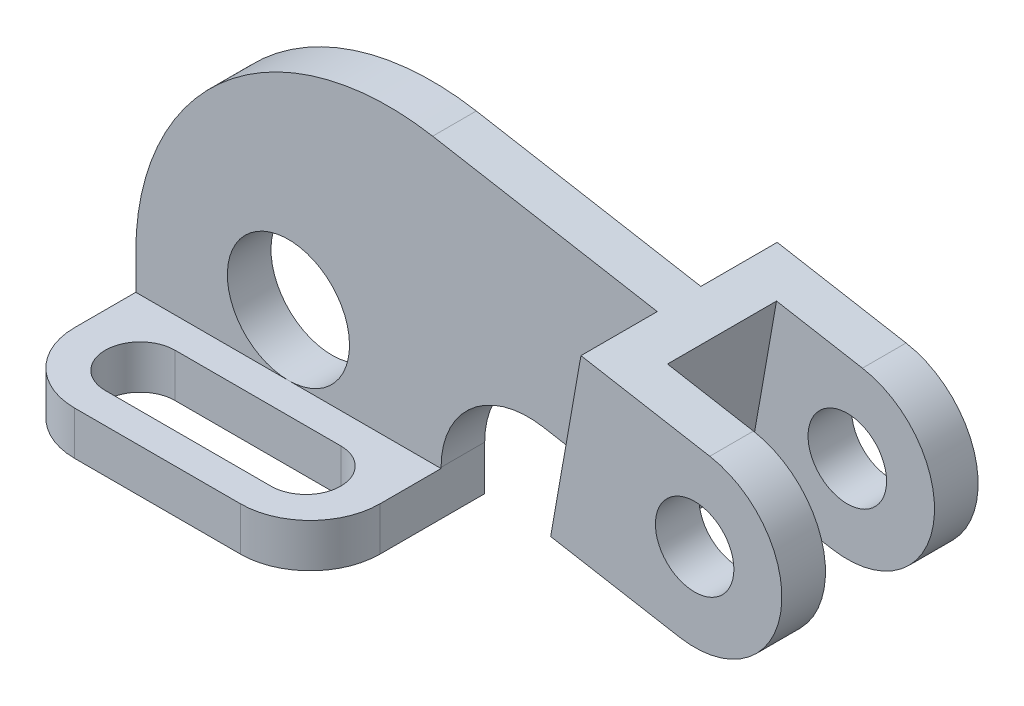
ISO-10303-21;
HEADER;
FILE_DESCRIPTION(('STEP AP214'),'2;1');
FILE_NAME('part.step','',(''),(''),'','','');
FILE_SCHEMA(('AUTOMOTIVE_DESIGN { 1 0 10303 214 1 1 1 1 }'));
ENDSEC;
DATA;
#1=APPLICATION_CONTEXT('core data for automotive mechanical design processes');
#2=APPLICATION_PROTOCOL_DEFINITION('international standard','automotive_design',2000,#1);
#3=PRODUCT_CONTEXT('',#1,'mechanical');
#4=PRODUCT('Part','Part','',(#3));
#5=PRODUCT_RELATED_PRODUCT_CATEGORY('part','',(#4));
#6=PRODUCT_DEFINITION_FORMATION('','',#4);
#7=PRODUCT_DEFINITION_CONTEXT('part definition',#1,'design');
#8=PRODUCT_DEFINITION('design','',#6,#7);
#9=PRODUCT_DEFINITION_SHAPE('','',#8);
#10=(LENGTH_UNIT() NAMED_UNIT(*) SI_UNIT(.MILLI.,.METRE.));
#11=(NAMED_UNIT(*) PLANE_ANGLE_UNIT() SI_UNIT($,.RADIAN.));
#12=(NAMED_UNIT(*) SI_UNIT($,.STERADIAN.) SOLID_ANGLE_UNIT());
#13=UNCERTAINTY_MEASURE_WITH_UNIT(LENGTH_MEASURE(1.E-05),#10,'distance_accuracy_value','');
#14=(GEOMETRIC_REPRESENTATION_CONTEXT(3) GLOBAL_UNCERTAINTY_ASSIGNED_CONTEXT((#13)) GLOBAL_UNIT_ASSIGNED_CONTEXT((#10,
#11,#12)) REPRESENTATION_CONTEXT('',''));
#15=CARTESIAN_POINT('',(0.,0.,0.));
#16=DIRECTION('',(0.,0.,1.));
#17=DIRECTION('',(1.,0.,0.));
#18=AXIS2_PLACEMENT_3D('',#15,#16,#17);
#19=CARTESIAN_POINT('',(145.640956215304,41.0463722757444,22.5));
#20=DIRECTION('',(0.,0.,1.));
#21=DIRECTION('',(1.,0.,0.));
#22=AXIS2_PLACEMENT_3D('',#19,#20,#21);
#23=CYLINDRICAL_SURFACE('',#22,20.);
#24=CARTESIAN_POINT('',(145.640956215304,41.0463722757444,-12.5));
#25=DIRECTION('',(0.,0.,-1.));
#26=DIRECTION('',(-1.,0.,0.));
#27=AXIS2_PLACEMENT_3D('',#24,#25,#26);
#28=CIRCLE('',#27,20.);
#29=CARTESIAN_POINT('',(142.167992661965,21.3502172155003,-12.5));
#30=VERTEX_POINT('',#29);
#31=CARTESIAN_POINT('',(149.113919768642,60.7425273359886,-12.5));
#32=VERTEX_POINT('',#31);
#33=EDGE_CURVE('E242',#30,#32,#28,.F.);
#34=ORIENTED_EDGE('',*,*,#33,.F.);
#35=DIRECTION('',(0.,0.,-1.));
#36=VECTOR('',#35,1.);
#37=CARTESIAN_POINT('',(142.167992661965,21.3502172155003,22.5));
#38=LINE('',#37,#36);
#39=CARTESIAN_POINT('',(142.167992661965,21.3502172155003,-22.5));
#40=VERTEX_POINT('',#39);
#41=EDGE_CURVE('E399',#40,#30,#38,.F.);
#42=ORIENTED_EDGE('',*,*,#41,.F.);
#43=CARTESIAN_POINT('',(145.640956215304,41.0463722757444,-22.5));
#44=DIRECTION('',(0.,0.,1.));
#45=DIRECTION('',(0.,-1.,0.));
#46=AXIS2_PLACEMENT_3D('',#43,#44,#45);
#47=CIRCLE('',#46,20.);
#48=CARTESIAN_POINT('',(149.113919768642,60.7425273359886,-22.5));
#49=VERTEX_POINT('',#48);
#50=EDGE_CURVE('E11',#49,#40,#47,.F.);
#51=ORIENTED_EDGE('',*,*,#50,.F.);
#52=DIRECTION('',(0.,0.,-1.));
#53=VECTOR('',#52,1.);
#54=CARTESIAN_POINT('',(149.113919768642,60.7425273359886,22.5));
#55=LINE('',#54,#53);
#56=EDGE_CURVE('E398',#32,#49,#55,.T.);
#57=ORIENTED_EDGE('',*,*,#56,.F.);
#58=EDGE_LOOP('',(#34,#42,#51,#57));
#59=FACE_BOUND('',#58,.T.);
#60=ADVANCED_FACE('F41',(#59),#23,.T.);
#61=CARTESIAN_POINT('',(68.0715943046827,75.0324758946416,5.));
#62=DIRECTION('',(-0.173648177666934,-0.984807753012207,0.));
#63=DIRECTION('',(0.984807753012207,-0.173648177666934,0.));
#64=AXIS2_PLACEMENT_3D('',#61,#62,#63);
#65=PLANE('',#64);
#66=DIRECTION('',(0.984807753012207,-0.173648177666934,0.));
#67=VECTOR('',#66,1.);
#68=CARTESIAN_POINT('',(129.417764708398,64.2154908893273,12.5));
#69=LINE('',#68,#67);
#70=CARTESIAN_POINT('',(129.417764708398,64.2154908893273,12.5));
#71=VERTEX_POINT('',#70);
#72=CARTESIAN_POINT('',(149.113919768642,60.7425273359886,12.5));
#73=VERTEX_POINT('',#72);
#74=EDGE_CURVE('E213',#71,#73,#69,.T.);
#75=ORIENTED_EDGE('',*,*,#74,.F.);
#76=DIRECTION('',(0.,0.,1.));
#77=VECTOR('',#76,1.);
#78=CARTESIAN_POINT('',(129.417764708398,64.2154908893273,-12.5));
#79=LINE('',#78,#77);
#80=CARTESIAN_POINT('',(129.417764708398,64.2154908893273,-12.5));
#81=VERTEX_POINT('',#80);
#82=EDGE_CURVE('E222',#81,#71,#79,.T.);
#83=ORIENTED_EDGE('',*,*,#82,.F.);
#84=DIRECTION('',(-0.984807753012207,0.173648177666934,0.));
#85=VECTOR('',#84,1.);
#86=CARTESIAN_POINT('',(129.417764708398,64.2154908893273,-12.5));
#87=LINE('',#86,#85);
#88=EDGE_CURVE('E56',#32,#81,#87,.T.);
#89=ORIENTED_EDGE('',*,*,#88,.F.);
#90=ORIENTED_EDGE('',*,*,#56,.T.);
#91=DIRECTION('',(-0.984807753012207,0.173648177666934,0.));
#92=VECTOR('',#91,1.);
#93=CARTESIAN_POINT('',(168.810074828886,57.2695637826499,-22.5));
#94=LINE('',#93,#92);
#95=CARTESIAN_POINT('',(119.569687178276,65.9519726659966,-22.5));
#96=VERTEX_POINT('',#95);
#97=EDGE_CURVE('E264',#49,#96,#94,.T.);
#98=ORIENTED_EDGE('',*,*,#97,.T.);
#99=DIRECTION('',(0.,0.,1.));
#100=VECTOR('',#99,1.);
#101=CARTESIAN_POINT('',(119.569687178276,65.9519726659966,22.5));
#102=LINE('',#101,#100);
#103=CARTESIAN_POINT('',(119.569687178276,65.9519726659966,-5.));
#104=VERTEX_POINT('',#103);
#105=EDGE_CURVE('E257',#96,#104,#102,.T.);
#106=ORIENTED_EDGE('',*,*,#105,.T.);
#107=DIRECTION('',(-0.984807753012207,0.173648177666934,0.));
#108=VECTOR('',#107,1.);
#109=CARTESIAN_POINT('',(68.0715943046827,75.0324758946416,-5.));
#110=LINE('',#109,#108);
#111=CARTESIAN_POINT('',(68.0715943046827,75.0324758946416,-5.));
#112=VERTEX_POINT('',#111);
#113=EDGE_CURVE('E373',#104,#112,#110,.T.);
#114=ORIENTED_EDGE('',*,*,#113,.T.);
#115=DIRECTION('',(0.,0.,-1.));
#116=VECTOR('',#115,1.);
#117=CARTESIAN_POINT('',(68.0715943046827,75.0324758946416,5.));
#118=LINE('',#117,#116);
#119=CARTESIAN_POINT('',(68.0715943046827,75.0324758946416,5.));
#120=VERTEX_POINT('',#119);
#121=EDGE_CURVE('E382',#120,#112,#118,.T.);
#122=ORIENTED_EDGE('',*,*,#121,.F.);
#123=DIRECTION('',(-0.984807753012207,0.173648177666934,0.));
#124=VECTOR('',#123,1.);
#125=CARTESIAN_POINT('',(68.0715943046827,75.0324758946416,5.));
#126=LINE('',#125,#124);
#127=CARTESIAN_POINT('',(119.569687178276,65.9519726659966,5.));
#128=VERTEX_POINT('',#127);
#129=EDGE_CURVE('E351',#128,#120,#126,.T.);
#130=ORIENTED_EDGE('',*,*,#129,.F.);
#131=CARTESIAN_POINT('',(119.569687178276,65.9519726659966,22.5));
#132=VERTEX_POINT('',#131);
#133=EDGE_CURVE('E259',#128,#132,#102,.T.);
#134=ORIENTED_EDGE('',*,*,#133,.T.);
#135=DIRECTION('',(-0.984807753012207,0.173648177666934,0.));
#136=VECTOR('',#135,1.);
#137=CARTESIAN_POINT('',(168.810074828886,57.2695637826499,22.5));
#138=LINE('',#137,#136);
#139=CARTESIAN_POINT('',(149.113919768642,60.7425273359886,22.5));
#140=VERTEX_POINT('',#139);
#141=EDGE_CURVE('E263',#140,#132,#138,.T.);
#142=ORIENTED_EDGE('',*,*,#141,.F.);
#143=EDGE_CURVE('E229',#140,#73,#55,.T.);
#144=ORIENTED_EDGE('',*,*,#143,.T.);
#145=EDGE_LOOP('',(#75,#83,#89,#90,#98,#106,#114,#122,#130,#134,#142,#144));
#146=FACE_BOUND('',#145,.T.);
#147=ADVANCED_FACE('F227',(#146),#65,.F.);
#148=CARTESIAN_POINT('',(145.640956215304,41.0463722757444,-27.5));
#149=DIRECTION('',(0.,0.,1.));
#150=DIRECTION('',(1.,0.,0.));
#151=AXIS2_PLACEMENT_3D('',#148,#149,#150);
#152=CYLINDRICAL_SURFACE('',#151,9.00000000000001);
#153=CARTESIAN_POINT('',(145.640956215304,41.0463722757444,-12.5));
#154=DIRECTION('',(0.,0.,-1.));
#155=DIRECTION('',(-1.,0.,0.));
#156=AXIS2_PLACEMENT_3D('',#153,#154,#155);
#157=CIRCLE('',#156,9.00000000000001);
#158=CARTESIAN_POINT('',(154.640956215304,41.0463722757444,-12.5));
#159=VERTEX_POINT('',#158);
#160=EDGE_CURVE('E46',#159,#159,#157,.F.);
#161=CARTESIAN_POINT('',(145.640956215304,41.0463722757444,-22.5));
#162=DIRECTION('',(0.,0.,1.));
#163=DIRECTION('',(0.,-1.,0.));
#164=AXIS2_PLACEMENT_3D('',#161,#162,#163);
#165=CIRCLE('',#164,9.00000000000001);
#166=CARTESIAN_POINT('',(154.640956215304,41.0463722757444,-22.5));
#167=VERTEX_POINT('',#166);
#168=EDGE_CURVE('E247',#167,#167,#165,.T.);
#169=CARTESIAN_POINT('',(154.640956215304,41.0463722757444,-12.5));
#170=CARTESIAN_POINT('',(154.640956215304,41.0463722757444,-12.6041666666667));
#171=CARTESIAN_POINT('',(154.640956215304,41.0463722757444,-12.7083333333333));
#172=CARTESIAN_POINT('',(154.640956215304,41.0463722757444,-12.9166666666667));
#173=CARTESIAN_POINT('',(154.640956215304,41.0463722757444,-13.0208333333333));
#174=CARTESIAN_POINT('',(154.640956215304,41.0463722757444,-13.2291666666667));
#175=CARTESIAN_POINT('',(154.640956215304,41.0463722757444,-13.3333333333333));
#176=CARTESIAN_POINT('',(154.640956215304,41.0463722757444,-13.5416666666667));
#177=CARTESIAN_POINT('',(154.640956215304,41.0463722757444,-13.6458333333333));
#178=CARTESIAN_POINT('',(154.640956215304,41.0463722757444,-13.8541666666667));
#179=CARTESIAN_POINT('',(154.640956215304,41.0463722757444,-13.9583333333333));
#180=CARTESIAN_POINT('',(154.640956215304,41.0463722757444,-14.1666666666667));
#181=CARTESIAN_POINT('',(154.640956215304,41.0463722757444,-14.2708333333333));
#182=CARTESIAN_POINT('',(154.640956215304,41.0463722757444,-14.4791666666667));
#183=CARTESIAN_POINT('',(154.640956215304,41.0463722757444,-14.5833333333333));
#184=CARTESIAN_POINT('',(154.640956215304,41.0463722757444,-14.7916666666667));
#185=CARTESIAN_POINT('',(154.640956215304,41.0463722757444,-14.8958333333333));
#186=CARTESIAN_POINT('',(154.640956215304,41.0463722757444,-15.1041666666667));
#187=CARTESIAN_POINT('',(154.640956215304,41.0463722757444,-15.2083333333333));
#188=CARTESIAN_POINT('',(154.640956215304,41.0463722757444,-15.4166666666667));
#189=CARTESIAN_POINT('',(154.640956215304,41.0463722757444,-15.5208333333333));
#190=CARTESIAN_POINT('',(154.640956215304,41.0463722757444,-15.7291666666667));
#191=CARTESIAN_POINT('',(154.640956215304,41.0463722757444,-15.8333333333333));
#192=CARTESIAN_POINT('',(154.640956215304,41.0463722757444,-16.0416666666667));
#193=CARTESIAN_POINT('',(154.640956215304,41.0463722757444,-16.1458333333333));
#194=CARTESIAN_POINT('',(154.640956215304,41.0463722757444,-16.3541666666667));
#195=CARTESIAN_POINT('',(154.640956215304,41.0463722757444,-16.4583333333333));
#196=CARTESIAN_POINT('',(154.640956215304,41.0463722757444,-16.6666666666667));
#197=CARTESIAN_POINT('',(154.640956215304,41.0463722757444,-16.7708333333333));
#198=CARTESIAN_POINT('',(154.640956215304,41.0463722757444,-16.9791666666667));
#199=CARTESIAN_POINT('',(154.640956215304,41.0463722757444,-17.0833333333333));
#200=CARTESIAN_POINT('',(154.640956215304,41.0463722757444,-17.2916666666667));
#201=CARTESIAN_POINT('',(154.640956215304,41.0463722757444,-17.3958333333333));
#202=CARTESIAN_POINT('',(154.640956215304,41.0463722757444,-17.6041666666667));
#203=CARTESIAN_POINT('',(154.640956215304,41.0463722757444,-17.7083333333333));
#204=CARTESIAN_POINT('',(154.640956215304,41.0463722757444,-17.9166666666667));
#205=CARTESIAN_POINT('',(154.640956215304,41.0463722757444,-18.0208333333333));
#206=CARTESIAN_POINT('',(154.640956215304,41.0463722757444,-18.2291666666667));
#207=CARTESIAN_POINT('',(154.640956215304,41.0463722757444,-18.3333333333333));
#208=CARTESIAN_POINT('',(154.640956215304,41.0463722757444,-18.5416666666667));
#209=CARTESIAN_POINT('',(154.640956215304,41.0463722757444,-18.6458333333333));
#210=CARTESIAN_POINT('',(154.640956215304,41.0463722757444,-18.8541666666667));
#211=CARTESIAN_POINT('',(154.640956215304,41.0463722757444,-18.9583333333333));
#212=CARTESIAN_POINT('',(154.640956215304,41.0463722757444,-19.1666666666667));
#213=CARTESIAN_POINT('',(154.640956215304,41.0463722757444,-19.2708333333333));
#214=CARTESIAN_POINT('',(154.640956215304,41.0463722757444,-19.4791666666667));
#215=CARTESIAN_POINT('',(154.640956215304,41.0463722757444,-19.5833333333333));
#216=CARTESIAN_POINT('',(154.640956215304,41.0463722757444,-19.7916666666667));
#217=CARTESIAN_POINT('',(154.640956215304,41.0463722757444,-19.8958333333333));
#218=CARTESIAN_POINT('',(154.640956215304,41.0463722757444,-20.1041666666667));
#219=CARTESIAN_POINT('',(154.640956215304,41.0463722757444,-20.2083333333333));
#220=CARTESIAN_POINT('',(154.640956215304,41.0463722757444,-20.4166666666667));
#221=CARTESIAN_POINT('',(154.640956215304,41.0463722757444,-20.5208333333333));
#222=CARTESIAN_POINT('',(154.640956215304,41.0463722757444,-20.7291666666667));
#223=CARTESIAN_POINT('',(154.640956215304,41.0463722757444,-20.8333333333333));
#224=CARTESIAN_POINT('',(154.640956215304,41.0463722757444,-21.0416666666667));
#225=CARTESIAN_POINT('',(154.640956215304,41.0463722757444,-21.1458333333333));
#226=CARTESIAN_POINT('',(154.640956215304,41.0463722757444,-21.3541666666667));
#227=CARTESIAN_POINT('',(154.640956215304,41.0463722757444,-21.4583333333333));
#228=CARTESIAN_POINT('',(154.640956215304,41.0463722757444,-21.6666666666667));
#229=CARTESIAN_POINT('',(154.640956215304,41.0463722757444,-21.7708333333333));
#230=CARTESIAN_POINT('',(154.640956215304,41.0463722757444,-21.9791666666667));
#231=CARTESIAN_POINT('',(154.640956215304,41.0463722757444,-22.0833333333333));
#232=CARTESIAN_POINT('',(154.640956215304,41.0463722757444,-22.2916666666667));
#233=CARTESIAN_POINT('',(154.640956215304,41.0463722757444,-22.3958333333333));
#234=CARTESIAN_POINT('',(154.640956215304,41.0463722757444,-22.5));
#235=B_SPLINE_CURVE_WITH_KNOTS('',3,(#169,#170,#171,#172,#173,#174,#175,#176,#177,#178,#179,
#180,#181,#182,#183,#184,#185,#186,#187,#188,#189,#190,#191,#192,#193,#194,#195,#196,#197,#198,
#199,#200,#201,#202,#203,#204,#205,#206,#207,#208,#209,#210,#211,#212,#213,#214,#215,#216,#217,
#218,#219,#220,#221,#222,#223,#224,#225,#226,#227,#228,#229,#230,#231,#232,#233,#234),
.UNSPECIFIED.,.F.,.F.,(4,2,2,2,2,2,2,2,2,2,2,2,2,2,2,2,2,2,2,2,2,2,2,2,2,2,2,2,2,2,2,2,4),(0.,
0.3125,0.625000000000001,0.937500000000001,1.25,1.5625,1.875,2.1875,2.5,2.8125,3.125,3.4375,
3.75,4.0625,4.375,4.6875,5.,5.3125,5.62500000000001,5.93750000000001,6.25000000000001,
6.56250000000001,6.87500000000001,7.18750000000001,7.5,7.8125,8.125,8.4375,8.75,
9.06250000000001,9.37500000000001,9.68750000000001,10.),.UNSPECIFIED.);
#236=EDGE_CURVE('BSEAM423',#159,#167,#235,.T.);
#237=ORIENTED_EDGE('',*,*,#160,.T.);
#238=ORIENTED_EDGE('',*,*,#168,.F.);
#239=ORIENTED_EDGE('',*,*,#236,.T.);
#240=ORIENTED_EDGE('',*,*,#236,.F.);
#241=EDGE_LOOP('',(#237,#239,#238,#240));
#242=FACE_BOUND('',#241,.T.);
#243=ADVANCED_FACE('F423',(#242),#152,.F.);
#244=CARTESIAN_POINT('',(145.640956215304,41.0463722757444,12.5));
#245=DIRECTION('',(0.,0.,1.));
#246=DIRECTION('',(1.,0.,0.));
#247=AXIS2_PLACEMENT_3D('',#244,#245,#246);
#248=CIRCLE('',#247,20.);
#249=CARTESIAN_POINT('',(142.167992661965,21.3502172155003,12.5));
#250=VERTEX_POINT('',#249);
#251=EDGE_CURVE('E237',#73,#250,#248,.F.);
#252=ORIENTED_EDGE('',*,*,#251,.F.);
#253=ORIENTED_EDGE('',*,*,#143,.F.);
#254=CARTESIAN_POINT('',(145.640956215304,41.0463722757444,22.5));
#255=DIRECTION('',(0.,0.,-1.));
#256=DIRECTION('',(0.,1.,0.));
#257=AXIS2_PLACEMENT_3D('',#254,#255,#256);
#258=CIRCLE('',#257,20.);
#259=CARTESIAN_POINT('',(142.167992661965,21.3502172155003,22.5));
#260=VERTEX_POINT('',#259);
#261=EDGE_CURVE('E51',#260,#140,#258,.F.);
#262=ORIENTED_EDGE('',*,*,#261,.F.);
#263=EDGE_CURVE('E69',#250,#260,#38,.F.);
#264=ORIENTED_EDGE('',*,*,#263,.F.);
#265=EDGE_LOOP('',(#252,#253,#262,#264));
#266=FACE_BOUND('',#265,.T.);
#267=ADVANCED_FACE('F42',(#266),#23,.T.);
#268=CARTESIAN_POINT('',(58.,17.9136262199337,5.));
#269=DIRECTION('',(0.,0.,1.));
#270=DIRECTION('',(1.,0.,0.));
#271=AXIS2_PLACEMENT_3D('',#268,#269,#270);
#272=PLANE('',#271);
#273=DIRECTION('',(-1.,0.,0.));
#274=VECTOR('',#273,1.);
#275=CARTESIAN_POINT('',(0.,10.,5.));
#276=LINE('',#275,#274);
#277=CARTESIAN_POINT('',(70.,10.,5.));
#278=VERTEX_POINT('',#277);
#279=CARTESIAN_POINT('',(35.,10.,5.));
#280=VERTEX_POINT('',#279);
#281=EDGE_CURVE('E316',#278,#280,#276,.T.);
#282=ORIENTED_EDGE('',*,*,#281,.F.);
#283=DIRECTION('',(0.,1.,0.));
#284=VECTOR('',#283,1.);
#285=CARTESIAN_POINT('',(70.,10.240309613491,5.));
#286=LINE('',#285,#284);
#287=CARTESIAN_POINT('',(70.,10.240309613491,5.));
#288=VERTEX_POINT('',#287);
#289=EDGE_CURVE('E345',#278,#288,#286,.T.);
#290=ORIENTED_EDGE('',*,*,#289,.T.);
#291=CARTESIAN_POINT('',(90.,10.2403096134912,5.));
#292=DIRECTION('',(0.,0.,-1.));
#293=DIRECTION('',(1.,0.,0.));
#294=AXIS2_PLACEMENT_3D('',#291,#292,#293);
#295=CIRCLE('',#294,20.);
#296=CARTESIAN_POINT('',(93.4729635533388,29.9364646737353,5.));
#297=VERTEX_POINT('',#296);
#298=EDGE_CURVE('E347',#288,#297,#295,.T.);
#299=ORIENTED_EDGE('',*,*,#298,.T.);
#300=DIRECTION('',(0.984807753012207,-0.173648177666934,0.));
#301=VECTOR('',#300,1.);
#302=CARTESIAN_POINT('',(112.623760071599,26.5596625455083,5.));
#303=LINE('',#302,#301);
#304=CARTESIAN_POINT('',(112.623760071599,26.5596625455083,5.00000000000001));
#305=VERTEX_POINT('',#304);
#306=EDGE_CURVE('E349',#297,#305,#303,.T.);
#307=ORIENTED_EDGE('',*,*,#306,.T.);
#308=DIRECTION('',(0.173648177666934,0.984807753012207,0.));
#309=VECTOR('',#308,1.);
#310=CARTESIAN_POINT('',(119.569687178276,65.9519726659966,5.));
#311=LINE('',#310,#309);
#312=EDGE_CURVE('E355',#305,#128,#311,.T.);
#313=ORIENTED_EDGE('',*,*,#312,.T.);
#314=ORIENTED_EDGE('',*,*,#129,.T.);
#315=CARTESIAN_POINT('',(58.,17.9136262199337,5.));
#316=DIRECTION('',(0.,0.,1.));
#317=DIRECTION('',(1.,0.,0.));
#318=AXIS2_PLACEMENT_3D('',#315,#316,#317);
#319=CIRCLE('',#318,58.);
#320=CARTESIAN_POINT('',(0.,17.9136262199332,5.));
#321=VERTEX_POINT('',#320);
#322=EDGE_CURVE('E359',#120,#321,#319,.T.);
#323=ORIENTED_EDGE('',*,*,#322,.T.);
#324=DIRECTION('',(0.,-1.,0.));
#325=VECTOR('',#324,1.);
#326=CARTESIAN_POINT('',(0.,0.,5.));
#327=LINE('',#326,#325);
#328=CARTESIAN_POINT('',(0.,10.,5.));
#329=VERTEX_POINT('',#328);
#330=EDGE_CURVE('E360',#321,#329,#327,.T.);
#331=ORIENTED_EDGE('',*,*,#330,.T.);
#332=EDGE_CURVE('E319',#280,#329,#276,.T.);
#333=ORIENTED_EDGE('',*,*,#332,.F.);
#334=CARTESIAN_POINT('',(35.,24.,5.));
#335=DIRECTION('',(0.,0.,1.));
#336=DIRECTION('',(1.,0.,0.));
#337=AXIS2_PLACEMENT_3D('',#334,#335,#336);
#338=CIRCLE('',#337,14.);
#339=EDGE_CURVE('E338',#280,#280,#338,.T.);
#340=ORIENTED_EDGE('',*,*,#339,.F.);
#341=EDGE_LOOP('',(#282,#290,#299,#307,#313,#314,#323,#331,#333,#340));
#342=FACE_BOUND('',#341,.T.);
#343=ADVANCED_FACE('F422',(#342),#272,.T.);
#344=CARTESIAN_POINT('',(58.,17.9136262199337,-5.));
#345=DIRECTION('',(0.,0.,1.));
#346=DIRECTION('',(1.,0.,0.));
#347=AXIS2_PLACEMENT_3D('',#344,#345,#346);
#348=PLANE('',#347);
#349=DIRECTION('',(1.,0.,0.));
#350=VECTOR('',#349,1.);
#351=CARTESIAN_POINT('',(70.,0.,-5.));
#352=LINE('',#351,#350);
#353=CARTESIAN_POINT('',(0.,0.,-5.));
#354=VERTEX_POINT('',#353);
#355=CARTESIAN_POINT('',(70.,0.,-5.));
#356=VERTEX_POINT('',#355);
#357=EDGE_CURVE('E343',#354,#356,#352,.T.);
#358=ORIENTED_EDGE('',*,*,#357,.F.);
#359=DIRECTION('',(0.,-1.,0.));
#360=VECTOR('',#359,1.);
#361=CARTESIAN_POINT('',(0.,0.,-5.));
#362=LINE('',#361,#360);
#363=CARTESIAN_POINT('',(0.,17.9136262199332,-5.));
#364=VERTEX_POINT('',#363);
#365=EDGE_CURVE('E350',#364,#354,#362,.T.);
#366=ORIENTED_EDGE('',*,*,#365,.F.);
#367=CARTESIAN_POINT('',(58.,17.9136262199337,-5.));
#368=DIRECTION('',(0.,0.,1.));
#369=DIRECTION('',(1.,0.,0.));
#370=AXIS2_PLACEMENT_3D('',#367,#368,#369);
#371=CIRCLE('',#370,58.);
#372=EDGE_CURVE('E374',#112,#364,#371,.T.);
#373=ORIENTED_EDGE('',*,*,#372,.F.);
#374=ORIENTED_EDGE('',*,*,#113,.F.);
#375=DIRECTION('',(0.173648177666934,0.984807753012207,0.));
#376=VECTOR('',#375,1.);
#377=CARTESIAN_POINT('',(119.569687178276,65.9519726659966,-5.));
#378=LINE('',#377,#376);
#379=CARTESIAN_POINT('',(112.623760071599,26.5596625455083,-4.99999999999999));
#380=VERTEX_POINT('',#379);
#381=EDGE_CURVE('E371',#380,#104,#378,.T.);
#382=ORIENTED_EDGE('',*,*,#381,.F.);
#383=DIRECTION('',(0.984807753012207,-0.173648177666934,0.));
#384=VECTOR('',#383,1.);
#385=CARTESIAN_POINT('',(112.623760071599,26.5596625455083,-5.));
#386=LINE('',#385,#384);
#387=CARTESIAN_POINT('',(93.4729635533388,29.9364646737353,-5.));
#388=VERTEX_POINT('',#387);
#389=EDGE_CURVE('E366',#388,#380,#386,.T.);
#390=ORIENTED_EDGE('',*,*,#389,.F.);
#391=CARTESIAN_POINT('',(90.,10.2403096134912,-5.));
#392=DIRECTION('',(0.,0.,-1.));
#393=DIRECTION('',(1.,0.,0.));
#394=AXIS2_PLACEMENT_3D('',#391,#392,#393);
#395=CIRCLE('',#394,20.);
#396=CARTESIAN_POINT('',(70.,10.240309613491,-5.));
#397=VERTEX_POINT('',#396);
#398=EDGE_CURVE('E368',#397,#388,#395,.T.);
#399=ORIENTED_EDGE('',*,*,#398,.F.);
#400=DIRECTION('',(0.,1.,0.));
#401=VECTOR('',#400,1.);
#402=CARTESIAN_POINT('',(70.,10.240309613491,-5.));
#403=LINE('',#402,#401);
#404=EDGE_CURVE('E365',#356,#397,#403,.T.);
#405=ORIENTED_EDGE('',*,*,#404,.F.);
#406=EDGE_LOOP('',(#358,#366,#373,#374,#382,#390,#399,#405));
#407=FACE_BOUND('',#406,.T.);
#408=CARTESIAN_POINT('',(35.,24.,-5.));
#409=DIRECTION('',(0.,0.,1.));
#410=DIRECTION('',(1.,0.,0.));
#411=AXIS2_PLACEMENT_3D('',#408,#409,#410);
#412=CIRCLE('',#411,14.);
#413=CARTESIAN_POINT('',(49.,24.,-5.));
#414=VERTEX_POINT('',#413);
#415=EDGE_CURVE('E340',#414,#414,#412,.T.);
#416=ORIENTED_EDGE('',*,*,#415,.T.);
#417=EDGE_LOOP('',(#416));
#418=FACE_BOUND('',#417,.T.);
#419=ADVANCED_FACE('F435',(#407,#418),#348,.F.);
#420=CARTESIAN_POINT('',(70.,0.,5.));
#421=DIRECTION('',(0.,1.,0.));
#422=DIRECTION('',(0.,0.,1.));
#423=AXIS2_PLACEMENT_3D('',#420,#421,#422);
#424=PLANE('',#423);
#425=ORIENTED_EDGE('',*,*,#357,.T.);
#426=DIRECTION('',(0.,0.,-1.));
#427=VECTOR('',#426,1.);
#428=CARTESIAN_POINT('',(70.,0.,5.));
#429=LINE('',#428,#427);
#430=CARTESIAN_POINT('',(70.,0.,19.));
#431=VERTEX_POINT('',#430);
#432=EDGE_CURVE('E395',#431,#356,#429,.T.);
#433=ORIENTED_EDGE('',*,*,#432,.F.);
#434=CARTESIAN_POINT('',(54.,0.,19.));
#435=DIRECTION('',(0.,1.,0.));
#436=DIRECTION('',(0.,0.,-1.));
#437=AXIS2_PLACEMENT_3D('',#434,#435,#436);
#438=CIRCLE('',#437,16.);
#439=CARTESIAN_POINT('',(54.,0.,35.));
#440=VERTEX_POINT('',#439);
#441=EDGE_CURVE('E307',#440,#431,#438,.T.);
#442=ORIENTED_EDGE('',*,*,#441,.F.);
#443=DIRECTION('',(1.,0.,0.));
#444=VECTOR('',#443,1.);
#445=CARTESIAN_POINT('',(16.,0.,35.));
#446=LINE('',#445,#444);
#447=CARTESIAN_POINT('',(16.,0.,35.));
#448=VERTEX_POINT('',#447);
#449=EDGE_CURVE('E325',#448,#440,#446,.T.);
#450=ORIENTED_EDGE('',*,*,#449,.F.);
#451=CARTESIAN_POINT('',(16.,0.,19.));
#452=DIRECTION('',(0.,1.,0.));
#453=DIRECTION('',(0.,0.,-1.));
#454=AXIS2_PLACEMENT_3D('',#451,#452,#453);
#455=CIRCLE('',#454,16.);
#456=CARTESIAN_POINT('',(0.,0.,19.));
#457=VERTEX_POINT('',#456);
#458=EDGE_CURVE('E304',#457,#448,#455,.T.);
#459=ORIENTED_EDGE('',*,*,#458,.F.);
#460=DIRECTION('',(0.,0.,-1.));
#461=VECTOR('',#460,1.);
#462=CARTESIAN_POINT('',(0.,0.,5.));
#463=LINE('',#462,#461);
#464=EDGE_CURVE('E363',#457,#354,#463,.T.);
#465=ORIENTED_EDGE('',*,*,#464,.T.);
#466=EDGE_LOOP('',(#425,#433,#442,#450,#459,#465));
#467=FACE_BOUND('',#466,.T.);
#468=DIRECTION('',(-1.,0.,0.));
#469=VECTOR('',#468,1.);
#470=CARTESIAN_POINT('',(16.,0.,12.));
#471=LINE('',#470,#469);
#472=CARTESIAN_POINT('',(54.,0.,12.));
#473=VERTEX_POINT('',#472);
#474=CARTESIAN_POINT('',(16.,0.,12.));
#475=VERTEX_POINT('',#474);
#476=EDGE_CURVE('E274',#473,#475,#471,.T.);
#477=ORIENTED_EDGE('',*,*,#476,.T.);
#478=CARTESIAN_POINT('',(16.,0.,20.));
#479=DIRECTION('',(0.,1.,0.));
#480=DIRECTION('',(0.,0.,1.));
#481=AXIS2_PLACEMENT_3D('',#478,#479,#480);
#482=CIRCLE('',#481,8.);
#483=CARTESIAN_POINT('',(16.,0.,28.));
#484=VERTEX_POINT('',#483);
#485=EDGE_CURVE('E271',#475,#484,#482,.T.);
#486=ORIENTED_EDGE('',*,*,#485,.T.);
#487=DIRECTION('',(1.,0.,0.));
#488=VECTOR('',#487,1.);
#489=CARTESIAN_POINT('',(16.,0.,28.));
#490=LINE('',#489,#488);
#491=CARTESIAN_POINT('',(54.,0.,28.));
#492=VERTEX_POINT('',#491);
#493=EDGE_CURVE('E281',#484,#492,#490,.T.);
#494=ORIENTED_EDGE('',*,*,#493,.T.);
#495=CARTESIAN_POINT('',(54.,0.,20.));
#496=DIRECTION('',(0.,1.,0.));
#497=DIRECTION('',(0.,0.,1.));
#498=AXIS2_PLACEMENT_3D('',#495,#496,#497);
#499=CIRCLE('',#498,8.);
#500=EDGE_CURVE('E287',#492,#473,#499,.T.);
#501=ORIENTED_EDGE('',*,*,#500,.T.);
#502=EDGE_LOOP('',(#477,#486,#494,#501));
#503=FACE_BOUND('',#502,.T.);
#504=ADVANCED_FACE('F487',(#467,#503),#424,.F.);
#505=CARTESIAN_POINT('',(70.,10.240309613491,5.));
#506=DIRECTION('',(-1.,0.,0.));
#507=DIRECTION('',(0.,0.,1.));
#508=AXIS2_PLACEMENT_3D('',#505,#506,#507);
#509=PLANE('',#508);
#510=ORIENTED_EDGE('',*,*,#404,.T.);
#511=DIRECTION('',(0.,0.,-1.));
#512=VECTOR('',#511,1.);
#513=CARTESIAN_POINT('',(70.,10.240309613491,5.));
#514=LINE('',#513,#512);
#515=EDGE_CURVE('E386',#288,#397,#514,.T.);
#516=ORIENTED_EDGE('',*,*,#515,.F.);
#517=ORIENTED_EDGE('',*,*,#289,.F.);
#518=DIRECTION('',(0.,0.,-1.));
#519=VECTOR('',#518,1.);
#520=CARTESIAN_POINT('',(70.,10.,5.));
#521=LINE('',#520,#519);
#522=CARTESIAN_POINT('',(70.,10.,19.));
#523=VERTEX_POINT('',#522);
#524=EDGE_CURVE('E311',#523,#278,#521,.T.);
#525=ORIENTED_EDGE('',*,*,#524,.F.);
#526=DIRECTION('',(0.,-1.,0.));
#527=VECTOR('',#526,1.);
#528=CARTESIAN_POINT('',(70.,10.,19.));
#529=LINE('',#528,#527);
#530=EDGE_CURVE('E317',#523,#431,#529,.T.);
#531=ORIENTED_EDGE('',*,*,#530,.T.);
#532=ORIENTED_EDGE('',*,*,#432,.T.);
#533=EDGE_LOOP('',(#510,#516,#517,#525,#531,#532));
#534=FACE_BOUND('',#533,.T.);
#535=ADVANCED_FACE('F480',(#534),#509,.F.);
#536=CARTESIAN_POINT('',(90.,10.2403096134912,5.));
#537=DIRECTION('',(0.,0.,-1.));
#538=DIRECTION('',(-1.,0.,0.));
#539=AXIS2_PLACEMENT_3D('',#536,#537,#538);
#540=CYLINDRICAL_SURFACE('',#539,20.);
#541=ORIENTED_EDGE('',*,*,#398,.T.);
#542=DIRECTION('',(0.,0.,-1.));
#543=VECTOR('',#542,1.);
#544=CARTESIAN_POINT('',(93.4729635533388,29.9364646737353,5.));
#545=LINE('',#544,#543);
#546=EDGE_CURVE('E387',#297,#388,#545,.T.);
#547=ORIENTED_EDGE('',*,*,#546,.F.);
#548=ORIENTED_EDGE('',*,*,#298,.F.);
#549=ORIENTED_EDGE('',*,*,#515,.T.);
#550=EDGE_LOOP('',(#541,#547,#548,#549));
#551=FACE_BOUND('',#550,.T.);
#552=ADVANCED_FACE('F508',(#551),#540,.F.);
#553=CARTESIAN_POINT('',(112.623760071599,26.5596625455083,5.));
#554=DIRECTION('',(0.173648177666934,0.984807753012207,0.));
#555=DIRECTION('',(-0.984807753012208,0.173648177666934,0.));
#556=AXIS2_PLACEMENT_3D('',#553,#554,#555);
#557=PLANE('',#556);
#558=ORIENTED_EDGE('',*,*,#41,.T.);
#559=DIRECTION('',(-0.984807753012207,0.173648177666934,0.));
#560=VECTOR('',#559,1.);
#561=CARTESIAN_POINT('',(112.623760071599,26.5596625455083,-12.5));
#562=LINE('',#561,#560);
#563=CARTESIAN_POINT('',(122.471837601721,24.823180768839,-12.5));
#564=VERTEX_POINT('',#563);
#565=EDGE_CURVE('E236',#30,#564,#562,.T.);
#566=ORIENTED_EDGE('',*,*,#565,.T.);
#567=DIRECTION('',(0.,0.,1.));
#568=VECTOR('',#567,1.);
#569=CARTESIAN_POINT('',(122.471837601721,24.8231807688389,5.));
#570=LINE('',#569,#568);
#571=CARTESIAN_POINT('',(122.471837601721,24.823180768839,12.5));
#572=VERTEX_POINT('',#571);
#573=EDGE_CURVE('E243',#564,#572,#570,.T.);
#574=ORIENTED_EDGE('',*,*,#573,.T.);
#575=DIRECTION('',(0.984807753012207,-0.173648177666934,0.));
#576=VECTOR('',#575,1.);
#577=CARTESIAN_POINT('',(112.623760071599,26.5596625455083,12.5));
#578=LINE('',#577,#576);
#579=EDGE_CURVE('E214',#572,#250,#578,.T.);
#580=ORIENTED_EDGE('',*,*,#579,.T.);
#581=ORIENTED_EDGE('',*,*,#263,.T.);
#582=DIRECTION('',(-0.984807753012207,0.173648177666934,0.));
#583=VECTOR('',#582,1.);
#584=CARTESIAN_POINT('',(161.864147722209,17.8772536621616,22.5));
#585=LINE('',#584,#583);
#586=CARTESIAN_POINT('',(112.623760071599,26.5596625455083,22.5));
#587=VERTEX_POINT('',#586);
#588=EDGE_CURVE('E267',#260,#587,#585,.T.);
#589=ORIENTED_EDGE('',*,*,#588,.T.);
#590=DIRECTION('',(0.,0.,-1.));
#591=VECTOR('',#590,1.);
#592=CARTESIAN_POINT('',(112.623760071599,26.5596625455083,22.5));
#593=LINE('',#592,#591);
#594=EDGE_CURVE('E251',#587,#305,#593,.T.);
#595=ORIENTED_EDGE('',*,*,#594,.T.);
#596=ORIENTED_EDGE('',*,*,#306,.F.);
#597=ORIENTED_EDGE('',*,*,#546,.T.);
#598=ORIENTED_EDGE('',*,*,#389,.T.);
#599=CARTESIAN_POINT('',(112.623760071599,26.5596625455083,-22.5));
#600=VERTEX_POINT('',#599);
#601=EDGE_CURVE('E252',#380,#600,#593,.T.);
#602=ORIENTED_EDGE('',*,*,#601,.T.);
#603=DIRECTION('',(-0.984807753012207,0.173648177666934,0.));
#604=VECTOR('',#603,1.);
#605=CARTESIAN_POINT('',(161.864147722209,17.8772536621616,-22.5));
#606=LINE('',#605,#604);
#607=EDGE_CURVE('E270',#40,#600,#606,.T.);
#608=ORIENTED_EDGE('',*,*,#607,.F.);
#609=EDGE_LOOP('',(#558,#566,#574,#580,#581,#589,#595,#596,#597,#598,#602,#608));
#610=FACE_BOUND('',#609,.T.);
#611=ADVANCED_FACE('F440',(#610),#557,.F.);
#612=CARTESIAN_POINT('',(58.,17.9136262199337,5.));
#613=DIRECTION('',(0.,0.,-1.));
#614=DIRECTION('',(-1.,0.,0.));
#615=AXIS2_PLACEMENT_3D('',#612,#613,#614);
#616=CYLINDRICAL_SURFACE('',#615,58.);
#617=ORIENTED_EDGE('',*,*,#372,.T.);
#618=DIRECTION('',(0.,0.,-1.));
#619=VECTOR('',#618,1.);
#620=CARTESIAN_POINT('',(0.,17.9136262199332,5.));
#621=LINE('',#620,#619);
#622=EDGE_CURVE('E379',#321,#364,#621,.T.);
#623=ORIENTED_EDGE('',*,*,#622,.F.);
#624=ORIENTED_EDGE('',*,*,#322,.F.);
#625=ORIENTED_EDGE('',*,*,#121,.T.);
#626=EDGE_LOOP('',(#617,#623,#624,#625));
#627=FACE_BOUND('',#626,.T.);
#628=ADVANCED_FACE('F502',(#627),#616,.T.);
#629=CARTESIAN_POINT('',(0.,0.,5.));
#630=DIRECTION('',(1.,0.,0.));
#631=DIRECTION('',(0.,1.,0.));
#632=AXIS2_PLACEMENT_3D('',#629,#630,#631);
#633=PLANE('',#632);
#634=ORIENTED_EDGE('',*,*,#365,.T.);
#635=ORIENTED_EDGE('',*,*,#464,.F.);
#636=DIRECTION('',(0.,-1.,0.));
#637=VECTOR('',#636,1.);
#638=CARTESIAN_POINT('',(0.,10.,19.));
#639=LINE('',#638,#637);
#640=CARTESIAN_POINT('',(0.,10.,19.));
#641=VERTEX_POINT('',#640);
#642=EDGE_CURVE('E331',#641,#457,#639,.T.);
#643=ORIENTED_EDGE('',*,*,#642,.F.);
#644=DIRECTION('',(0.,0.,1.));
#645=VECTOR('',#644,1.);
#646=CARTESIAN_POINT('',(0.,10.,5.));
#647=LINE('',#646,#645);
#648=EDGE_CURVE('E302',#329,#641,#647,.T.);
#649=ORIENTED_EDGE('',*,*,#648,.F.);
#650=ORIENTED_EDGE('',*,*,#330,.F.);
#651=ORIENTED_EDGE('',*,*,#622,.T.);
#652=EDGE_LOOP('',(#634,#635,#643,#649,#650,#651));
#653=FACE_BOUND('',#652,.T.);
#654=ADVANCED_FACE('F459',(#653),#633,.F.);
#655=CARTESIAN_POINT('',(35.,24.,5.));
#656=DIRECTION('',(0.,0.,-1.));
#657=DIRECTION('',(-1.,0.,0.));
#658=AXIS2_PLACEMENT_3D('',#655,#656,#657);
#659=CYLINDRICAL_SURFACE('',#658,14.);
#660=ORIENTED_EDGE('',*,*,#339,.T.);
#661=EDGE_LOOP('',(#660));
#662=FACE_BOUND('',#661,.T.);
#663=ORIENTED_EDGE('',*,*,#415,.F.);
#664=EDGE_LOOP('',(#663));
#665=FACE_BOUND('',#664,.T.);
#666=ADVANCED_FACE('F485',(#662,#665),#659,.F.);
#667=CARTESIAN_POINT('',(16.,10.,19.));
#668=DIRECTION('',(0.,-1.,0.));
#669=DIRECTION('',(0.,0.,-1.));
#670=AXIS2_PLACEMENT_3D('',#667,#668,#669);
#671=PLANE('',#670);
#672=ORIENTED_EDGE('',*,*,#648,.T.);
#673=CARTESIAN_POINT('',(16.,10.,19.));
#674=DIRECTION('',(0.,1.,0.));
#675=DIRECTION('',(0.,0.,-1.));
#676=AXIS2_PLACEMENT_3D('',#673,#674,#675);
#677=CIRCLE('',#676,16.);
#678=CARTESIAN_POINT('',(16.,10.,35.));
#679=VERTEX_POINT('',#678);
#680=EDGE_CURVE('E308',#641,#679,#677,.T.);
#681=ORIENTED_EDGE('',*,*,#680,.T.);
#682=DIRECTION('',(1.,0.,0.));
#683=VECTOR('',#682,1.);
#684=CARTESIAN_POINT('',(16.,10.,35.));
#685=LINE('',#684,#683);
#686=CARTESIAN_POINT('',(54.,10.,35.));
#687=VERTEX_POINT('',#686);
#688=EDGE_CURVE('E310',#679,#687,#685,.T.);
#689=ORIENTED_EDGE('',*,*,#688,.T.);
#690=CARTESIAN_POINT('',(54.,10.,19.));
#691=DIRECTION('',(0.,1.,0.));
#692=DIRECTION('',(0.,0.,-1.));
#693=AXIS2_PLACEMENT_3D('',#690,#691,#692);
#694=CIRCLE('',#693,16.);
#695=EDGE_CURVE('E313',#687,#523,#694,.T.);
#696=ORIENTED_EDGE('',*,*,#695,.T.);
#697=ORIENTED_EDGE('',*,*,#524,.T.);
#698=ORIENTED_EDGE('',*,*,#281,.T.);
#699=ORIENTED_EDGE('',*,*,#332,.T.);
#700=EDGE_LOOP('',(#672,#681,#689,#696,#697,#698,#699));
#701=FACE_BOUND('',#700,.T.);
#702=CARTESIAN_POINT('',(16.,10.,20.));
#703=DIRECTION('',(0.,1.,0.));
#704=DIRECTION('',(0.,0.,1.));
#705=AXIS2_PLACEMENT_3D('',#702,#703,#704);
#706=CIRCLE('',#705,8.);
#707=CARTESIAN_POINT('',(16.,10.,12.));
#708=VERTEX_POINT('',#707);
#709=CARTESIAN_POINT('',(16.,10.,28.));
#710=VERTEX_POINT('',#709);
#711=EDGE_CURVE('E275',#708,#710,#706,.T.);
#712=ORIENTED_EDGE('',*,*,#711,.F.);
#713=DIRECTION('',(-1.,0.,0.));
#714=VECTOR('',#713,1.);
#715=CARTESIAN_POINT('',(16.,10.,12.));
#716=LINE('',#715,#714);
#717=CARTESIAN_POINT('',(54.,10.,12.));
#718=VERTEX_POINT('',#717);
#719=EDGE_CURVE('E278',#718,#708,#716,.T.);
#720=ORIENTED_EDGE('',*,*,#719,.F.);
#721=CARTESIAN_POINT('',(54.,10.,20.));
#722=DIRECTION('',(0.,1.,0.));
#723=DIRECTION('',(0.,0.,1.));
#724=AXIS2_PLACEMENT_3D('',#721,#722,#723);
#725=CIRCLE('',#724,8.);
#726=CARTESIAN_POINT('',(54.,10.,28.));
#727=VERTEX_POINT('',#726);
#728=EDGE_CURVE('E280',#727,#718,#725,.T.);
#729=ORIENTED_EDGE('',*,*,#728,.F.);
#730=DIRECTION('',(1.,0.,0.));
#731=VECTOR('',#730,1.);
#732=CARTESIAN_POINT('',(16.,10.,28.));
#733=LINE('',#732,#731);
#734=EDGE_CURVE('E273',#710,#727,#733,.T.);
#735=ORIENTED_EDGE('',*,*,#734,.F.);
#736=EDGE_LOOP('',(#712,#720,#729,#735));
#737=FACE_BOUND('',#736,.T.);
#738=ADVANCED_FACE('F452',(#701,#737),#671,.F.);
#739=CARTESIAN_POINT('',(16.,10.,19.));
#740=DIRECTION('',(0.,-1.,0.));
#741=DIRECTION('',(0.,0.,-1.));
#742=AXIS2_PLACEMENT_3D('',#739,#740,#741);
#743=CYLINDRICAL_SURFACE('',#742,16.);
#744=ORIENTED_EDGE('',*,*,#458,.T.);
#745=DIRECTION('',(0.,-1.,0.));
#746=VECTOR('',#745,1.);
#747=CARTESIAN_POINT('',(16.,10.,35.));
#748=LINE('',#747,#746);
#749=EDGE_CURVE('E332',#679,#448,#748,.T.);
#750=ORIENTED_EDGE('',*,*,#749,.F.);
#751=ORIENTED_EDGE('',*,*,#680,.F.);
#752=ORIENTED_EDGE('',*,*,#642,.T.);
#753=EDGE_LOOP('',(#744,#750,#751,#752));
#754=FACE_BOUND('',#753,.T.);
#755=ADVANCED_FACE('F465',(#754),#743,.T.);
#756=CARTESIAN_POINT('',(16.,10.,35.));
#757=DIRECTION('',(0.,0.,-1.));
#758=DIRECTION('',(-1.,0.,0.));
#759=AXIS2_PLACEMENT_3D('',#756,#757,#758);
#760=PLANE('',#759);
#761=ORIENTED_EDGE('',*,*,#449,.T.);
#762=DIRECTION('',(0.,-1.,0.));
#763=VECTOR('',#762,1.);
#764=CARTESIAN_POINT('',(54.,10.,35.));
#765=LINE('',#764,#763);
#766=EDGE_CURVE('E327',#687,#440,#765,.T.);
#767=ORIENTED_EDGE('',*,*,#766,.F.);
#768=ORIENTED_EDGE('',*,*,#688,.F.);
#769=ORIENTED_EDGE('',*,*,#749,.T.);
#770=EDGE_LOOP('',(#761,#767,#768,#769));
#771=FACE_BOUND('',#770,.T.);
#772=ADVANCED_FACE('F470',(#771),#760,.F.);
#773=CARTESIAN_POINT('',(54.,10.,19.));
#774=DIRECTION('',(0.,-1.,0.));
#775=DIRECTION('',(0.,0.,-1.));
#776=AXIS2_PLACEMENT_3D('',#773,#774,#775);
#777=CYLINDRICAL_SURFACE('',#776,16.);
#778=ORIENTED_EDGE('',*,*,#441,.T.);
#779=ORIENTED_EDGE('',*,*,#530,.F.);
#780=ORIENTED_EDGE('',*,*,#695,.F.);
#781=ORIENTED_EDGE('',*,*,#766,.T.);
#782=EDGE_LOOP('',(#778,#779,#780,#781));
#783=FACE_BOUND('',#782,.T.);
#784=ADVANCED_FACE('F471',(#783),#777,.T.);
#785=CARTESIAN_POINT('',(16.,10.,20.));
#786=DIRECTION('',(0.,-1.,0.));
#787=DIRECTION('',(0.,0.,-1.));
#788=AXIS2_PLACEMENT_3D('',#785,#786,#787);
#789=CYLINDRICAL_SURFACE('',#788,8.);
#790=ORIENTED_EDGE('',*,*,#485,.F.);
#791=DIRECTION('',(0.,-1.,0.));
#792=VECTOR('',#791,1.);
#793=CARTESIAN_POINT('',(16.,10.,12.));
#794=LINE('',#793,#792);
#795=EDGE_CURVE('E285',#708,#475,#794,.T.);
#796=ORIENTED_EDGE('',*,*,#795,.F.);
#797=ORIENTED_EDGE('',*,*,#711,.T.);
#798=DIRECTION('',(0.,-1.,0.));
#799=VECTOR('',#798,1.);
#800=CARTESIAN_POINT('',(16.,10.,28.));
#801=LINE('',#800,#799);
#802=EDGE_CURVE('E299',#710,#484,#801,.T.);
#803=ORIENTED_EDGE('',*,*,#802,.T.);
#804=EDGE_LOOP('',(#790,#796,#797,#803));
#805=FACE_BOUND('',#804,.T.);
#806=ADVANCED_FACE('F554',(#805),#789,.F.);
#807=CARTESIAN_POINT('',(16.,10.,28.));
#808=DIRECTION('',(0.,0.,-1.));
#809=DIRECTION('',(-1.,0.,0.));
#810=AXIS2_PLACEMENT_3D('',#807,#808,#809);
#811=PLANE('',#810);
#812=ORIENTED_EDGE('',*,*,#493,.F.);
#813=ORIENTED_EDGE('',*,*,#802,.F.);
#814=ORIENTED_EDGE('',*,*,#734,.T.);
#815=DIRECTION('',(0.,-1.,0.));
#816=VECTOR('',#815,1.);
#817=CARTESIAN_POINT('',(54.,10.,28.));
#818=LINE('',#817,#816);
#819=EDGE_CURVE('E300',#727,#492,#818,.T.);
#820=ORIENTED_EDGE('',*,*,#819,.T.);
#821=EDGE_LOOP('',(#812,#813,#814,#820));
#822=FACE_BOUND('',#821,.T.);
#823=ADVANCED_FACE('F563',(#822),#811,.T.);
#824=CARTESIAN_POINT('',(54.,10.,20.));
#825=DIRECTION('',(0.,-1.,0.));
#826=DIRECTION('',(0.,0.,-1.));
#827=AXIS2_PLACEMENT_3D('',#824,#825,#826);
#828=CYLINDRICAL_SURFACE('',#827,8.);
#829=ORIENTED_EDGE('',*,*,#500,.F.);
#830=ORIENTED_EDGE('',*,*,#819,.F.);
#831=ORIENTED_EDGE('',*,*,#728,.T.);
#832=DIRECTION('',(0.,-1.,0.));
#833=VECTOR('',#832,1.);
#834=CARTESIAN_POINT('',(54.,10.,12.));
#835=LINE('',#834,#833);
#836=EDGE_CURVE('E293',#718,#473,#835,.T.);
#837=ORIENTED_EDGE('',*,*,#836,.T.);
#838=EDGE_LOOP('',(#829,#830,#831,#837));
#839=FACE_BOUND('',#838,.T.);
#840=ADVANCED_FACE('F568',(#839),#828,.F.);
#841=CARTESIAN_POINT('',(16.,10.,12.));
#842=DIRECTION('',(0.,0.,1.));
#843=DIRECTION('',(1.,0.,0.));
#844=AXIS2_PLACEMENT_3D('',#841,#842,#843);
#845=PLANE('',#844);
#846=ORIENTED_EDGE('',*,*,#476,.F.);
#847=ORIENTED_EDGE('',*,*,#836,.F.);
#848=ORIENTED_EDGE('',*,*,#719,.T.);
#849=ORIENTED_EDGE('',*,*,#795,.T.);
#850=EDGE_LOOP('',(#846,#847,#848,#849));
#851=FACE_BOUND('',#850,.T.);
#852=ADVANCED_FACE('F580',(#851),#845,.T.);
#853=CARTESIAN_POINT('',(104.685768372773,-18.4589254603172,0.));
#854=DIRECTION('',(0.984807753012207,-0.173648177666934,0.));
#855=DIRECTION('',(0.173648177666934,0.984807753012207,0.));
#856=AXIS2_PLACEMENT_3D('',#853,#854,#855);
#857=PLANE('',#856);
#858=ORIENTED_EDGE('',*,*,#601,.F.);
#859=ORIENTED_EDGE('',*,*,#381,.T.);
#860=ORIENTED_EDGE('',*,*,#105,.F.);
#861=DIRECTION('',(0.173648177666934,0.984807753012207,0.));
#862=VECTOR('',#861,1.);
#863=CARTESIAN_POINT('',(119.569687178276,65.9519726659966,-22.5));
#864=LINE('',#863,#862);
#865=EDGE_CURVE('E258',#600,#96,#864,.T.);
#866=ORIENTED_EDGE('',*,*,#865,.F.);
#867=EDGE_LOOP('',(#858,#859,#860,#866));
#868=FACE_BOUND('',#867,.T.);
#869=ADVANCED_FACE('F590',(#868),#857,.F.);
#870=CARTESIAN_POINT('',(168.810074828886,57.2695637826499,22.5));
#871=DIRECTION('',(0.,0.,-1.));
#872=DIRECTION('',(0.,1.,0.));
#873=AXIS2_PLACEMENT_3D('',#870,#871,#872);
#874=PLANE('',#873);
#875=CARTESIAN_POINT('',(145.640956215304,41.0463722757444,22.5));
#876=DIRECTION('',(0.,0.,1.));
#877=DIRECTION('',(1.,0.,0.));
#878=AXIS2_PLACEMENT_3D('',#875,#876,#877);
#879=CIRCLE('',#878,9.00000000000001);
#880=CARTESIAN_POINT('',(154.640956215304,41.0463722757444,22.5));
#881=VERTEX_POINT('',#880);
#882=EDGE_CURVE('E241',#881,#881,#879,.T.);
#883=ORIENTED_EDGE('',*,*,#882,.F.);
#884=EDGE_LOOP('',(#883));
#885=FACE_BOUND('',#884,.T.);
#886=ORIENTED_EDGE('',*,*,#588,.F.);
#887=ORIENTED_EDGE('',*,*,#261,.T.);
#888=ORIENTED_EDGE('',*,*,#141,.T.);
#889=DIRECTION('',(-0.173648177666934,-0.984807753012207,0.));
#890=VECTOR('',#889,1.);
#891=CARTESIAN_POINT('',(119.569687178276,65.9519726659966,22.5));
#892=LINE('',#891,#890);
#893=EDGE_CURVE('E250',#132,#587,#892,.T.);
#894=ORIENTED_EDGE('',*,*,#893,.T.);
#895=EDGE_LOOP('',(#886,#887,#888,#894));
#896=FACE_BOUND('',#895,.T.);
#897=ADVANCED_FACE('F651',(#885,#896),#874,.F.);
#898=CARTESIAN_POINT('',(168.810074828886,57.2695637826499,-22.5));
#899=DIRECTION('',(0.,0.,1.));
#900=DIRECTION('',(0.,-1.,0.));
#901=AXIS2_PLACEMENT_3D('',#898,#899,#900);
#902=PLANE('',#901);
#903=ORIENTED_EDGE('',*,*,#168,.T.);
#904=EDGE_LOOP('',(#903));
#905=FACE_BOUND('',#904,.T.);
#906=ORIENTED_EDGE('',*,*,#97,.F.);
#907=ORIENTED_EDGE('',*,*,#50,.T.);
#908=ORIENTED_EDGE('',*,*,#607,.T.);
#909=ORIENTED_EDGE('',*,*,#865,.T.);
#910=EDGE_LOOP('',(#906,#907,#908,#909));
#911=FACE_BOUND('',#910,.T.);
#912=ADVANCED_FACE('F450',(#905,#911),#902,.F.);
#913=ORIENTED_EDGE('',*,*,#312,.F.);
#914=ORIENTED_EDGE('',*,*,#594,.F.);
#915=ORIENTED_EDGE('',*,*,#893,.F.);
#916=ORIENTED_EDGE('',*,*,#133,.F.);
#917=EDGE_LOOP('',(#913,#914,#915,#916));
#918=FACE_BOUND('',#917,.T.);
#919=ADVANCED_FACE('F652',(#918),#857,.F.);
#920=CARTESIAN_POINT('',(145.640956215304,41.0463722757444,12.5));
#921=DIRECTION('',(0.,0.,1.));
#922=DIRECTION('',(1.,0.,0.));
#923=AXIS2_PLACEMENT_3D('',#920,#921,#922);
#924=CIRCLE('',#923,9.00000000000001);
#925=CARTESIAN_POINT('',(154.640956215304,41.0463722757444,12.5));
#926=VERTEX_POINT('',#925);
#927=EDGE_CURVE('E232',#926,#926,#924,.F.);
#928=ORIENTED_EDGE('',*,*,#927,.T.);
#929=EDGE_LOOP('',(#928));
#930=FACE_BOUND('',#929,.T.);
#931=ORIENTED_EDGE('',*,*,#882,.T.);
#932=EDGE_LOOP('',(#931));
#933=FACE_BOUND('',#932,.T.);
#934=ADVANCED_FACE('F403',(#930,#933),#152,.F.);
#935=CARTESIAN_POINT('',(120.735355825051,14.9751032387169,-12.5));
#936=DIRECTION('',(-0.984807753012207,0.173648177666934,0.));
#937=DIRECTION('',(-0.173648177666934,-0.984807753012207,0.));
#938=AXIS2_PLACEMENT_3D('',#935,#936,#937);
#939=PLANE('',#938);
#940=DIRECTION('',(0.173648177666934,0.984807753012207,0.));
#941=VECTOR('',#940,1.);
#942=CARTESIAN_POINT('',(120.735355825051,14.9751032387169,-12.5));
#943=LINE('',#942,#941);
#944=EDGE_CURVE('E217',#564,#81,#943,.T.);
#945=ORIENTED_EDGE('',*,*,#944,.T.);
#946=ORIENTED_EDGE('',*,*,#82,.T.);
#947=DIRECTION('',(0.173648177666934,0.984807753012207,0.));
#948=VECTOR('',#947,1.);
#949=CARTESIAN_POINT('',(120.735355825051,14.9751032387169,12.5));
#950=LINE('',#949,#948);
#951=EDGE_CURVE('E208',#572,#71,#950,.T.);
#952=ORIENTED_EDGE('',*,*,#951,.F.);
#953=ORIENTED_EDGE('',*,*,#573,.F.);
#954=EDGE_LOOP('',(#945,#946,#952,#953));
#955=FACE_BOUND('',#954,.T.);
#956=ADVANCED_FACE('F225',(#955),#939,.F.);
#957=CARTESIAN_POINT('',(120.735355825051,14.9751032387169,-12.5));
#958=DIRECTION('',(0.,0.,-1.));
#959=DIRECTION('',(-1.,0.,0.));
#960=AXIS2_PLACEMENT_3D('',#957,#958,#959);
#961=PLANE('',#960);
#962=ORIENTED_EDGE('',*,*,#33,.T.);
#963=ORIENTED_EDGE('',*,*,#88,.T.);
#964=ORIENTED_EDGE('',*,*,#944,.F.);
#965=ORIENTED_EDGE('',*,*,#565,.F.);
#966=EDGE_LOOP('',(#962,#963,#964,#965));
#967=FACE_BOUND('',#966,.T.);
#968=ORIENTED_EDGE('',*,*,#160,.F.);
#969=EDGE_LOOP('',(#968));
#970=FACE_BOUND('',#969,.T.);
#971=ADVANCED_FACE('F408',(#967,#970),#961,.F.);
#972=CARTESIAN_POINT('',(120.735355825051,14.9751032387169,12.5));
#973=DIRECTION('',(0.,0.,1.));
#974=DIRECTION('',(1.,0.,0.));
#975=AXIS2_PLACEMENT_3D('',#972,#973,#974);
#976=PLANE('',#975);
#977=ORIENTED_EDGE('',*,*,#251,.T.);
#978=ORIENTED_EDGE('',*,*,#579,.F.);
#979=ORIENTED_EDGE('',*,*,#951,.T.);
#980=ORIENTED_EDGE('',*,*,#74,.T.);
#981=EDGE_LOOP('',(#977,#978,#979,#980));
#982=FACE_BOUND('',#981,.T.);
#983=ORIENTED_EDGE('',*,*,#927,.F.);
#984=EDGE_LOOP('',(#983));
#985=FACE_BOUND('',#984,.T.);
#986=ADVANCED_FACE('F209',(#982,#985),#976,.F.);
#987=CLOSED_SHELL('',(#60,#147,#243,#267,#343,#419,#504,#535,#552,#611,#628,#654,#666,#738,#755,
#772,#784,#806,#823,#840,#852,#869,#897,#912,#919,#934,#956,#971,#986));
#988=MANIFOLD_SOLID_BREP('B2',#987);
#989=ADVANCED_BREP_SHAPE_REPRESENTATION('',(#18,#988),#14);
#990=SHAPE_DEFINITION_REPRESENTATION(#9,#989);
ENDSEC;
END-ISO-10303-21;
